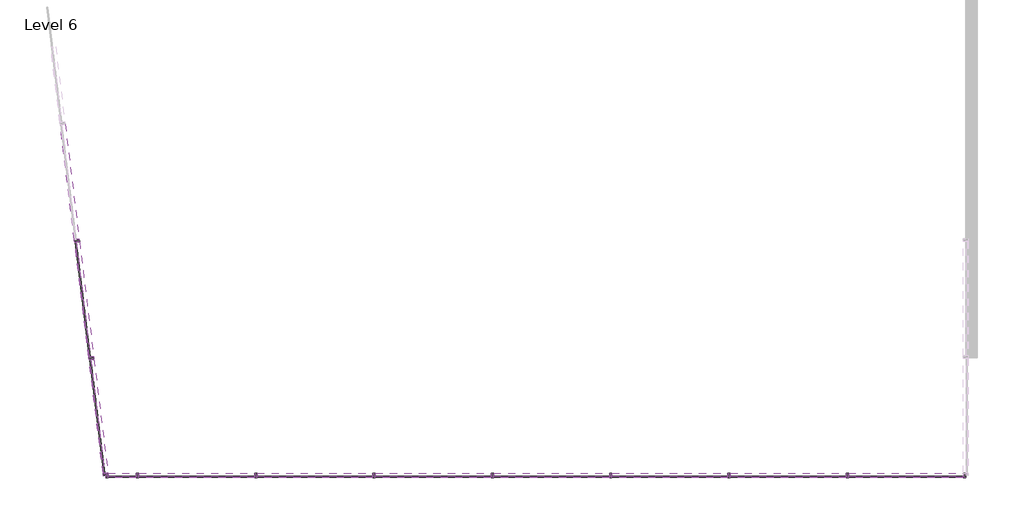
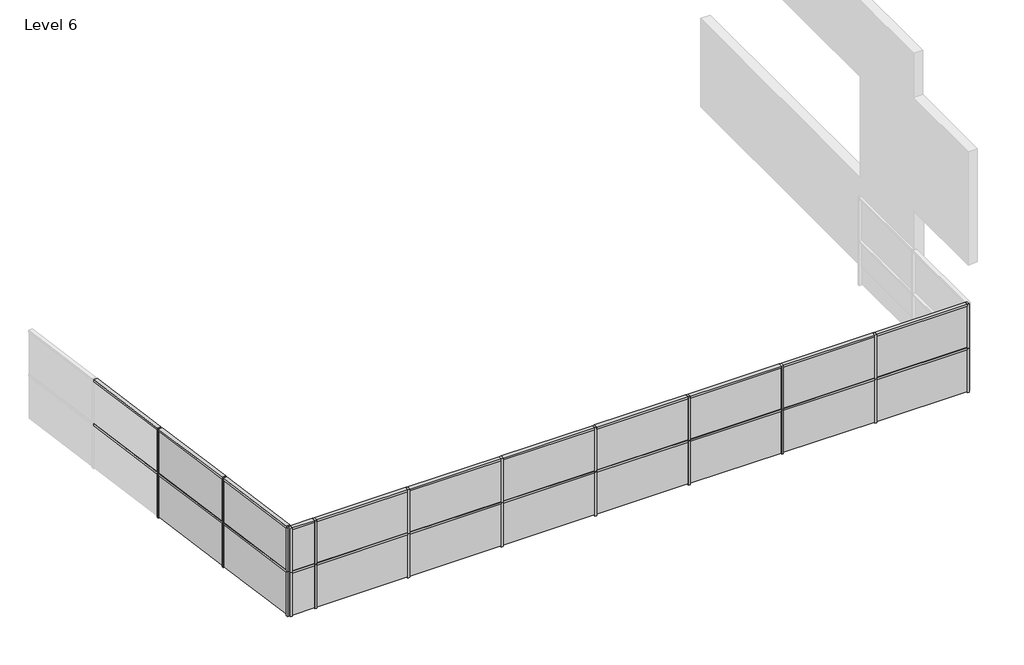
# One storey, part 1 of 2: 46 members, 20 plates.
"""IFC4 building model written with IfcOpenShell, lengths in millimetres."""

from ifc_helpers import new_model, si_unit, origin, place, context, project, spatial, transform, mapped, element, save
from components import member_daa7a266, member_82905deb, member_19d0a4ec, member_8cef0660, member_db480205, member_4491d118, member_0c11e56c, member_695b83e4, system_panel_glazed_37f15d2e, system_panel_glazed_3620f98e, system_panel_glazed_e46d4b42, system_panel_glazed_2a6c68b7, system_panel_glazed_07b088f8, system_panel_glazed_9d0e0944

model = new_model("IFC4")

# Units and contexts
model_context = context("Model", 3, world=origin())
ifc_project = project(units=[si_unit("LENGTHUNIT", "METRE", prefix="MILLI")], contexts=[model_context])

# Site, building, storey
site = spatial("IfcSite", under=ifc_project)
building = spatial("IfcBuilding", under=site)
storey = spatial("IfcBuildingStorey", under=building, Name="Level 6", Elevation=15240.0)

# Members
placement = place(None, origin())
member_shape = member_daa7a266(model_context)
element("IfcMember", 1, ObjectType="Rectangular Mullion : 2.5\" x 5\" rectangular", at=placement, inside=storey, context=model_context, shape_type="MappedRepresentation", body=[
    mapped(member_shape, transform((13839.0156363, -6979.1363705, 18288.0), x_axis=(0.0, 0.0, 1.0), y_axis=(0.0, -1.0, 0.0), z_axis=(1.0, 0.0, 0.0))),
])
member_2_shape = member_82905deb(model_context)
element("IfcMember", 2, ObjectType="Rectangular Mullion : 2.5\" x 5\" rectangular", at=placement, inside=storey, context=model_context, shape_type="MappedRepresentation", body=[
    mapped(member_2_shape, transform((10854.515636, -6979.1363705, 18288.0), x_axis=(-1.0, 0.0, 0.0), y_axis=(0.0, -1.0, 0.0), z_axis=(0.0, 0.0, 1.0))),
])
element("IfcMember", 3, ObjectType="Rectangular Mullion : 2.5\" x 5\" rectangular", at=placement, inside=storey, context=model_context, shape_type="MappedRepresentation", body=[
    mapped(member_2_shape, transform((7806.515636, -6979.1363705, 18288.0), x_axis=(-1.0, 0.0, 0.0), y_axis=(0.0, -1.0, 0.0), z_axis=(0.0, 0.0, 1.0))),
])
element("IfcMember", 4, ObjectType="Rectangular Mullion : 2.5\" x 5\" rectangular", at=placement, inside=storey, context=model_context, shape_type="MappedRepresentation", body=[
    mapped(member_2_shape, transform((4758.515636, -6979.1363705, 18288.0), x_axis=(-1.0, 0.0, 0.0), y_axis=(0.0, -1.0, 0.0), z_axis=(0.0, 0.0, 1.0))),
])
element("IfcMember", 5, ObjectType="Rectangular Mullion : 2.5\" x 5\" rectangular", at=placement, inside=storey, context=model_context, shape_type="MappedRepresentation", body=[
    mapped(member_2_shape, transform((1710.515636, -6979.1363705, 18288.0), x_axis=(-1.0, 0.0, 0.0), y_axis=(0.0, -1.0, 0.0), z_axis=(0.0, 0.0, 1.0))),
])
element("IfcMember", 6, ObjectType="Rectangular Mullion : 2.5\" x 5\" rectangular", at=placement, inside=storey, context=model_context, shape_type="MappedRepresentation", body=[
    mapped(member_2_shape, transform((-1337.484364, -6979.1363705, 18288.0), x_axis=(-1.0, 0.0, 0.0), y_axis=(0.0, -1.0, 0.0), z_axis=(0.0, 0.0, 1.0))),
])
element("IfcMember", 7, ObjectType="Rectangular Mullion : 2.5\" x 5\" rectangular", at=placement, inside=storey, context=model_context, shape_type="MappedRepresentation", body=[
    mapped(member_2_shape, transform((-4385.484364, -6979.1363705, 18288.0), x_axis=(-1.0, 0.0, 0.0), y_axis=(0.0, -1.0, 0.0), z_axis=(0.0, 0.0, 1.0))),
])
element("IfcMember", 8, ObjectType="Rectangular Mullion : 2.5\" x 5\" rectangular", at=placement, inside=storey, context=model_context, shape_type="MappedRepresentation", body=[
    mapped(member_2_shape, transform((-7433.484364, -6979.1363705, 18288.0), x_axis=(-1.0, 0.0, 0.0), y_axis=(0.0, -1.0, 0.0), z_axis=(0.0, 0.0, 1.0))),
])
member_3_shape = member_19d0a4ec(model_context)
element("IfcMember", 9, ObjectType="Rectangular Mullion : 2.5\" x 5\" rectangular", at=placement, inside=storey, context=model_context, shape_type="MappedRepresentation", body=[
    mapped(member_3_shape, transform((13839.0156363, -6979.1363705, 16764.0), x_axis=(0.0, 0.0, 1.0), y_axis=(0.0, -1.0, 0.0), z_axis=(1.0, 0.0, 0.0))),
])
element("IfcMember", 10, ObjectType="Rectangular Mullion : 2.5\" x 5\" rectangular", at=placement, inside=storey, context=model_context, shape_type="MappedRepresentation", body=[
    mapped(member_3_shape, transform((-8260.4765148, -6916.1096898, 16764.0), x_axis=(0.0, 0.0, 1.0), y_axis=(-0.9925461516413222, -0.12186934340514598, 0.0), z_axis=(0.12186934340514596, -0.9925461516413221, 0.0))),
])
element("IfcMember", 11, ObjectType="Rectangular Mullion : 2.5\" x 5\" rectangular", at=placement, inside=storey, context=model_context, shape_type="MappedRepresentation", body=[
    mapped(member_3_shape, transform((-8260.4765148, -6916.1096898, 18288.0), x_axis=(0.0, 0.0, 1.0), y_axis=(-0.9925461516413222, -0.12186934340514585, 0.0), z_axis=(0.12186934340514584, -0.9925461516413221, 0.0))),
])
member_4_shape = member_8cef0660(model_context)
element("IfcMember", 12, ObjectType="Rectangular Mullion : 2.5\" x 5\" rectangular", at=placement, inside=storey, context=model_context, shape_type="MappedRepresentation", body=[
    mapped(member_4_shape, transform((10822.765636, -6979.1363705, 16764.0), x_axis=(0.0, 0.0, 1.0), y_axis=(0.0, -1.0, 0.0), z_axis=(1.0, 0.0, 0.0))),
])
element("IfcMember", 13, ObjectType="Rectangular Mullion : 2.5\" x 5\" rectangular", at=placement, inside=storey, context=model_context, shape_type="MappedRepresentation", body=[
    mapped(member_4_shape, transform((7774.765636, -6979.1363705, 16764.0), x_axis=(0.0, 0.0, 1.0), y_axis=(0.0, -1.0, 0.0), z_axis=(1.0, 0.0, 0.0))),
])
element("IfcMember", 14, ObjectType="Rectangular Mullion : 2.5\" x 5\" rectangular", at=placement, inside=storey, context=model_context, shape_type="MappedRepresentation", body=[
    mapped(member_4_shape, transform((4726.765636, -6979.1363705, 16764.0), x_axis=(0.0, 0.0, 1.0), y_axis=(0.0, -1.0, 0.0), z_axis=(1.0, 0.0, 0.0))),
])
element("IfcMember", 15, ObjectType="Rectangular Mullion : 2.5\" x 5\" rectangular", at=placement, inside=storey, context=model_context, shape_type="MappedRepresentation", body=[
    mapped(member_4_shape, transform((1678.765636, -6979.1363705, 16764.0), x_axis=(0.0, 0.0, 1.0), y_axis=(0.0, -1.0, 0.0), z_axis=(1.0, 0.0, 0.0))),
])
element("IfcMember", 16, ObjectType="Rectangular Mullion : 2.5\" x 5\" rectangular", at=placement, inside=storey, context=model_context, shape_type="MappedRepresentation", body=[
    mapped(member_4_shape, transform((-1369.234364, -6979.1363705, 16764.0), x_axis=(0.0, 0.0, 1.0), y_axis=(0.0, -1.0, 0.0), z_axis=(1.0, 0.0, 0.0))),
])
element("IfcMember", 17, ObjectType="Rectangular Mullion : 2.5\" x 5\" rectangular", at=placement, inside=storey, context=model_context, shape_type="MappedRepresentation", body=[
    mapped(member_4_shape, transform((-4417.234364, -6979.1363705, 16764.0), x_axis=(0.0, 0.0, 1.0), y_axis=(0.0, -1.0, 0.0), z_axis=(1.0, 0.0, 0.0))),
])
element("IfcMember", 18, ObjectType="Rectangular Mullion : 2.5\" x 5\" rectangular", at=placement, inside=storey, context=model_context, shape_type="MappedRepresentation", body=[
    mapped(member_4_shape, transform((-8628.0649219, -3922.3423596, 16764.0), x_axis=(0.0, 0.0, 1.0), y_axis=(-0.9925461516413222, -0.12186934340514595, 0.0), z_axis=(0.12186934340514595, -0.9925461516413222, 0.0))),
])
element("IfcMember", 19, ObjectType="Rectangular Mullion : 2.5\" x 5\" rectangular", at=placement, inside=storey, context=model_context, shape_type="MappedRepresentation", body=[
    mapped(member_4_shape, transform((-8999.5226806, -897.0616894, 16764.0), x_axis=(0.0, 0.0, 1.0), y_axis=(-0.9925461516413222, -0.12186934340514602, 0.0), z_axis=(0.12186934340514602, -0.9925461516413222, 0.0))),
])
element("IfcMember", 20, ObjectType="Rectangular Mullion : 2.5\" x 5\" rectangular", at=placement, inside=storey, context=model_context, shape_type="MappedRepresentation", body=[
    mapped(member_4_shape, transform((-8628.0649219, -3922.3423596, 18288.0), x_axis=(0.0, 0.0, 1.0), y_axis=(-0.9925461516413222, -0.12186934340514595, 0.0), z_axis=(0.12186934340514595, -0.9925461516413222, 0.0))),
])
element("IfcMember", 21, ObjectType="Rectangular Mullion : 2.5\" x 5\" rectangular", at=placement, inside=storey, context=model_context, shape_type="MappedRepresentation", body=[
    mapped(member_4_shape, transform((-8999.5226806, -897.0616894, 18288.0), x_axis=(0.0, 0.0, 1.0), y_axis=(-0.9925461516413222, -0.12186934340514566, 0.0), z_axis=(0.12186934340514566, -0.9925461516413222, 0.0))),
])
member_5_shape = member_db480205(model_context)
element("IfcMember", 22, ObjectType="Rectangular Mullion : 2.5\" x 5\" rectangular", at=placement, inside=storey, context=model_context, shape_type="MappedRepresentation", body=[
    mapped(member_5_shape, transform((10822.765636, -6979.1363705, 18288.0), x_axis=(0.0, 0.0, 1.0), y_axis=(0.0, -1.0, 0.0), z_axis=(1.0, 0.0, 0.0))),
])
element("IfcMember", 23, ObjectType="Rectangular Mullion : 2.5\" x 5\" rectangular", at=placement, inside=storey, context=model_context, shape_type="MappedRepresentation", body=[
    mapped(member_5_shape, transform((7774.765636, -6979.1363705, 18288.0), x_axis=(0.0, 0.0, 1.0), y_axis=(0.0, -1.0, 0.0), z_axis=(1.0, 0.0, 0.0))),
])
element("IfcMember", 24, ObjectType="Rectangular Mullion : 2.5\" x 5\" rectangular", at=placement, inside=storey, context=model_context, shape_type="MappedRepresentation", body=[
    mapped(member_5_shape, transform((4726.765636, -6979.1363705, 18288.0), x_axis=(0.0, 0.0, 1.0), y_axis=(0.0, -1.0, 0.0), z_axis=(1.0, 0.0, 0.0))),
])
element("IfcMember", 25, ObjectType="Rectangular Mullion : 2.5\" x 5\" rectangular", at=placement, inside=storey, context=model_context, shape_type="MappedRepresentation", body=[
    mapped(member_5_shape, transform((1678.765636, -6979.1363705, 18288.0), x_axis=(0.0, 0.0, 1.0), y_axis=(0.0, -1.0, 0.0), z_axis=(1.0, 0.0, 0.0))),
])
element("IfcMember", 26, ObjectType="Rectangular Mullion : 2.5\" x 5\" rectangular", at=placement, inside=storey, context=model_context, shape_type="MappedRepresentation", body=[
    mapped(member_5_shape, transform((-1369.234364, -6979.1363705, 18288.0), x_axis=(0.0, 0.0, 1.0), y_axis=(0.0, -1.0, 0.0), z_axis=(1.0, 0.0, 0.0))),
])
element("IfcMember", 27, ObjectType="Rectangular Mullion : 2.5\" x 5\" rectangular", at=placement, inside=storey, context=model_context, shape_type="MappedRepresentation", body=[
    mapped(member_5_shape, transform((-4417.234364, -6979.1363705, 18288.0), x_axis=(0.0, 0.0, 1.0), y_axis=(0.0, -1.0, 0.0), z_axis=(1.0, 0.0, 0.0))),
])
element("IfcMember", 28, ObjectType="Rectangular Mullion : 2.5\" x 5\" rectangular", at=placement, inside=storey, context=model_context, shape_type="MappedRepresentation", body=[
    mapped(member_2_shape, transform((10854.515636, -6979.1363705, 16764.0), x_axis=(-1.0, 0.0, 0.0), y_axis=(0.0, -1.0, 0.0), z_axis=(0.0, 0.0, 1.0))),
])
element("IfcMember", 29, ObjectType="Rectangular Mullion : 2.5\" x 5\" rectangular", at=placement, inside=storey, context=model_context, shape_type="MappedRepresentation", body=[
    mapped(member_2_shape, transform((7806.515636, -6979.1363705, 16764.0), x_axis=(-1.0, 0.0, 0.0), y_axis=(0.0, -1.0, 0.0), z_axis=(0.0, 0.0, 1.0))),
])
element("IfcMember", 30, ObjectType="Rectangular Mullion : 2.5\" x 5\" rectangular", at=placement, inside=storey, context=model_context, shape_type="MappedRepresentation", body=[
    mapped(member_2_shape, transform((4758.515636, -6979.1363705, 16764.0), x_axis=(-1.0, 0.0, 0.0), y_axis=(0.0, -1.0, 0.0), z_axis=(0.0, 0.0, 1.0))),
])
element("IfcMember", 31, ObjectType="Rectangular Mullion : 2.5\" x 5\" rectangular", at=placement, inside=storey, context=model_context, shape_type="MappedRepresentation", body=[
    mapped(member_2_shape, transform((1710.515636, -6979.1363705, 16764.0), x_axis=(-1.0, 0.0, 0.0), y_axis=(0.0, -1.0, 0.0), z_axis=(0.0, 0.0, 1.0))),
])
element("IfcMember", 32, ObjectType="Rectangular Mullion : 2.5\" x 5\" rectangular", at=placement, inside=storey, context=model_context, shape_type="MappedRepresentation", body=[
    mapped(member_2_shape, transform((-1337.484364, -6979.1363705, 16764.0), x_axis=(-1.0, 0.0, 0.0), y_axis=(0.0, -1.0, 0.0), z_axis=(0.0, 0.0, 1.0))),
])
element("IfcMember", 33, ObjectType="Rectangular Mullion : 2.5\" x 5\" rectangular", at=placement, inside=storey, context=model_context, shape_type="MappedRepresentation", body=[
    mapped(member_2_shape, transform((-4385.484364, -6979.1363705, 16764.0), x_axis=(-1.0, 0.0, 0.0), y_axis=(0.0, -1.0, 0.0), z_axis=(0.0, 0.0, 1.0))),
])
element("IfcMember", 34, ObjectType="Rectangular Mullion : 2.5\" x 5\" rectangular", at=placement, inside=storey, context=model_context, shape_type="MappedRepresentation", body=[
    mapped(member_2_shape, transform((-7433.484364, -6979.1363705, 16764.0), x_axis=(-1.0, 0.0, 0.0), y_axis=(0.0, -1.0, 0.0), z_axis=(0.0, 0.0, 1.0))),
])
element("IfcMember", 35, ObjectType="Rectangular Mullion : 2.5\" x 5\" rectangular", at=placement, inside=storey, context=model_context, shape_type="MappedRepresentation", body=[
    mapped(member_2_shape, transform((-8624.1955702, -3953.8557, 16764.0), x_axis=(-0.1218693434051459, 0.9925461516413222, 0.0), y_axis=(-0.9925461516413222, -0.1218693434051459, 0.0), z_axis=(0.0, 0.0, 1.0))),
])
element("IfcMember", 36, ObjectType="Rectangular Mullion : 2.5\" x 5\" rectangular", at=placement, inside=storey, context=model_context, shape_type="MappedRepresentation", body=[
    mapped(member_2_shape, transform((-8624.1955702, -3953.8557, 18288.0), x_axis=(-0.1218693434051459, 0.9925461516413222, 0.0), y_axis=(-0.9925461516413222, -0.1218693434051459, 0.0), z_axis=(0.0, 0.0, 1.0))),
])
element("IfcMember", 37, ObjectType="Rectangular Mullion : 2.5\" x 5\" rectangular", at=placement, inside=storey, context=model_context, shape_type="MappedRepresentation", body=[
    mapped(member_2_shape, transform((-8995.6533289, -928.5750297, 16764.0), x_axis=(-0.1218693434051459, 0.9925461516413222, 0.0), y_axis=(-0.9925461516413222, -0.1218693434051459, 0.0), z_axis=(0.0, 0.0, 1.0))),
])
element("IfcMember", 38, ObjectType="Rectangular Mullion : 2.5\" x 5\" rectangular", at=placement, inside=storey, context=model_context, shape_type="MappedRepresentation", body=[
    mapped(member_2_shape, transform((-8995.6533289, -928.5750297, 18288.0), x_axis=(-0.1218693434051459, 0.9925461516413222, 0.0), y_axis=(-0.9925461516413222, -0.1218693434051459, 0.0), z_axis=(0.0, 0.0, 1.0))),
])
member_6_shape = member_4491d118(model_context)
element("IfcMember", 39, ObjectType="Rectangular Mullion : 2.5\" x 5\" rectangular", at=placement, inside=storey, context=model_context, shape_type="MappedRepresentation", body=[
    mapped(member_6_shape, transform((-8252.7378115, -6979.1363705, 18288.0), x_axis=(-1.0, 0.0, 0.0), y_axis=(0.0, -1.0, 0.0), z_axis=(0.0, 0.0, 1.0))),
])
element("IfcMember", 40, ObjectType="Rectangular Mullion : 2.5\" x 5\" rectangular", at=placement, inside=storey, context=model_context, shape_type="MappedRepresentation", body=[
    mapped(member_6_shape, transform((13902.5156363, -6979.1363705, 15240.0), x_axis=(1.0, 0.0, 0.0), y_axis=(0.0, -1.0, 0.0), z_axis=(0.0, 0.0, -1.0))),
])
element("IfcMember", 41, ObjectType="Rectangular Mullion : 2.5\" x 5\" rectangular", at=placement, inside=storey, context=model_context, shape_type="MappedRepresentation", body=[
    mapped(member_6_shape, transform((-8252.7378115, -6979.1363705, 15240.0), x_axis=(0.1218693434051459, -0.9925461516413222, 0.0), y_axis=(-0.9925461516413222, -0.1218693434051459, 0.0), z_axis=(0.0, 0.0, -1.0))),
])
element("IfcMember", 42, ObjectType="Rectangular Mullion : 2.5\" x 5\" rectangular", at=placement, inside=storey, context=model_context, shape_type="MappedRepresentation", body=[
    mapped(member_6_shape, transform((-8252.7378115, -6979.1363705, 16764.0), x_axis=(0.1218693434051459, -0.9925461516413222, 0.0), y_axis=(-0.9925461516413222, -0.1218693434051459, 0.0), z_axis=(0.0, 0.0, -1.0))),
])
element("IfcMember", 43, ObjectType="Rectangular Mullion : 2.5\" x 5\" rectangular", at=placement, inside=storey, context=model_context, shape_type="MappedRepresentation", body=[
    mapped(member_6_shape, transform((13902.5156363, -6979.1363705, 16764.0), x_axis=(1.0, 0.0, 0.0), y_axis=(0.0, -1.0, 0.0), z_axis=(0.0, 0.0, -1.0))),
])
element("IfcMember", 44, ObjectType="Rectangular Mullion : 2.5\" x 5\" rectangular", at=placement, inside=storey, context=model_context, shape_type="MappedRepresentation", body=[
    mapped(member_6_shape, transform((-8252.7378115, -6979.1363705, 16764.0), x_axis=(-1.0, 0.0, 0.0), y_axis=(0.0, -1.0, 0.0), z_axis=(0.0, 0.0, 1.0))),
])
member_7_shape = member_0c11e56c(model_context)
element("IfcMember", 45, ObjectType="Rectangular Mullion : 2.5\" x 5\" rectangular", at=placement, inside=storey, context=model_context, shape_type="MappedRepresentation", body=[
    mapped(member_7_shape, transform((-7465.234364, -6979.1363705, 16764.0), x_axis=(0.0, 0.0, 1.0), y_axis=(0.0, -1.0, 0.0), z_axis=(1.0, 0.0, 0.0))),
])
member_8_shape = member_695b83e4(model_context)
element("IfcMember", 46, ObjectType="Rectangular Mullion : 2.5\" x 5\" rectangular", at=placement, inside=storey, context=model_context, shape_type="MappedRepresentation", body=[
    mapped(member_8_shape, transform((-7465.234364, -6979.1363705, 18288.0), x_axis=(0.0, 0.0, 1.0), y_axis=(0.0, -1.0, 0.0), z_axis=(1.0, 0.0, 0.0))),
])

# Plates
system_panel_glazed_shape = system_panel_glazed_37f15d2e(model_context)
element("IfcPlate", 47, ObjectType="System Panel : Glazed", at=placement, inside=storey, context=model_context, shape_type="MappedRepresentation", body=[
    mapped(system_panel_glazed_shape, transform((12362.6406361, -6979.1363705, 16795.75), x_axis=(-1.0, 0.0, 0.0), y_axis=(0.0, -1.0, 0.0), z_axis=(0.0, 0.0, 1.0))),
])
system_panel_glazed_2_shape = system_panel_glazed_3620f98e(model_context)
element("IfcPlate", 48, ObjectType="System Panel : Glazed", at=placement, inside=storey, context=model_context, shape_type="MappedRepresentation", body=[
    mapped(system_panel_glazed_2_shape, transform((9330.515636, -6979.1363705, 16795.75), x_axis=(-1.0, 0.0, 0.0), y_axis=(0.0, -1.0, 0.0), z_axis=(0.0, 0.0, 1.0))),
])
element("IfcPlate", 49, ObjectType="System Panel : Glazed", at=placement, inside=storey, context=model_context, shape_type="MappedRepresentation", body=[
    mapped(system_panel_glazed_2_shape, transform((6282.515636, -6979.1363705, 16795.75), x_axis=(-1.0, 0.0, 0.0), y_axis=(0.0, -1.0, 0.0), z_axis=(0.0, 0.0, 1.0))),
])
element("IfcPlate", 50, ObjectType="System Panel : Glazed", at=placement, inside=storey, context=model_context, shape_type="MappedRepresentation", body=[
    mapped(system_panel_glazed_2_shape, transform((3234.515636, -6979.1363705, 16795.75), x_axis=(-1.0, 0.0, 0.0), y_axis=(0.0, -1.0, 0.0), z_axis=(0.0, 0.0, 1.0))),
])
element("IfcPlate", 51, ObjectType="System Panel : Glazed", at=placement, inside=storey, context=model_context, shape_type="MappedRepresentation", body=[
    mapped(system_panel_glazed_2_shape, transform((186.515636, -6979.1363705, 16795.75), x_axis=(-1.0, 0.0, 0.0), y_axis=(0.0, -1.0, 0.0), z_axis=(0.0, 0.0, 1.0))),
])
element("IfcPlate", 52, ObjectType="System Panel : Glazed", at=placement, inside=storey, context=model_context, shape_type="MappedRepresentation", body=[
    mapped(system_panel_glazed_2_shape, transform((-2861.484364, -6979.1363705, 16795.75), x_axis=(-1.0, 0.0, 0.0), y_axis=(0.0, -1.0, 0.0), z_axis=(0.0, 0.0, 1.0))),
])
element("IfcPlate", 53, ObjectType="System Panel : Glazed", at=placement, inside=storey, context=model_context, shape_type="MappedRepresentation", body=[
    mapped(system_panel_glazed_2_shape, transform((-5909.484364, -6979.1363705, 16795.75), x_axis=(-1.0, 0.0, 0.0), y_axis=(0.0, -1.0, 0.0), z_axis=(0.0, 0.0, 1.0))),
])
system_panel_glazed_3_shape = system_panel_glazed_e46d4b42(model_context)
element("IfcPlate", 54, ObjectType="System Panel : Glazed", at=placement, inside=storey, context=model_context, shape_type="MappedRepresentation", body=[
    mapped(system_panel_glazed_3_shape, transform((12362.6406361, -6979.1363705, 15271.75), x_axis=(-1.0, 0.0, 0.0), y_axis=(0.0, -1.0, 0.0), z_axis=(0.0, 0.0, 1.0))),
])
element("IfcPlate", 55, ObjectType="System Panel : Glazed", at=placement, inside=storey, context=model_context, shape_type="MappedRepresentation", body=[
    mapped(system_panel_glazed_3_shape, transform((-8440.4013667, -5450.739365, 15271.75), x_axis=(-0.1218693434051459, 0.9925461516413222, 0.0), y_axis=(-0.9925461516413222, -0.1218693434051459, 0.0), z_axis=(0.0, 0.0, 1.0))),
])
element("IfcPlate", 56, ObjectType="System Panel : Glazed", at=placement, inside=storey, context=model_context, shape_type="MappedRepresentation", body=[
    mapped(system_panel_glazed_3_shape, transform((-8440.4013667, -5450.739365, 16795.75), x_axis=(-0.1218693434051459, 0.9925461516413222, 0.0), y_axis=(-0.9925461516413222, -0.1218693434051459, 0.0), z_axis=(0.0, 0.0, 1.0))),
])
system_panel_glazed_4_shape = system_panel_glazed_2a6c68b7(model_context)
element("IfcPlate", 57, ObjectType="System Panel : Glazed", at=placement, inside=storey, context=model_context, shape_type="MappedRepresentation", body=[
    mapped(system_panel_glazed_4_shape, transform((9330.515636, -6979.1363705, 15271.75), x_axis=(-1.0, 0.0, 0.0), y_axis=(0.0, -1.0, 0.0), z_axis=(0.0, 0.0, 1.0))),
])
element("IfcPlate", 58, ObjectType="System Panel : Glazed", at=placement, inside=storey, context=model_context, shape_type="MappedRepresentation", body=[
    mapped(system_panel_glazed_4_shape, transform((6282.515636, -6979.1363705, 15271.75), x_axis=(-1.0, 0.0, 0.0), y_axis=(0.0, -1.0, 0.0), z_axis=(0.0, 0.0, 1.0))),
])
element("IfcPlate", 59, ObjectType="System Panel : Glazed", at=placement, inside=storey, context=model_context, shape_type="MappedRepresentation", body=[
    mapped(system_panel_glazed_4_shape, transform((3234.515636, -6979.1363705, 15271.75), x_axis=(-1.0, 0.0, 0.0), y_axis=(0.0, -1.0, 0.0), z_axis=(0.0, 0.0, 1.0))),
])
element("IfcPlate", 60, ObjectType="System Panel : Glazed", at=placement, inside=storey, context=model_context, shape_type="MappedRepresentation", body=[
    mapped(system_panel_glazed_4_shape, transform((186.515636, -6979.1363705, 15271.75), x_axis=(-1.0, 0.0, 0.0), y_axis=(0.0, -1.0, 0.0), z_axis=(0.0, 0.0, 1.0))),
])
element("IfcPlate", 61, ObjectType="System Panel : Glazed", at=placement, inside=storey, context=model_context, shape_type="MappedRepresentation", body=[
    mapped(system_panel_glazed_4_shape, transform((-2861.484364, -6979.1363705, 15271.75), x_axis=(-1.0, 0.0, 0.0), y_axis=(0.0, -1.0, 0.0), z_axis=(0.0, 0.0, 1.0))),
])
element("IfcPlate", 62, ObjectType="System Panel : Glazed", at=placement, inside=storey, context=model_context, shape_type="MappedRepresentation", body=[
    mapped(system_panel_glazed_4_shape, transform((-5909.484364, -6979.1363705, 15271.75), x_axis=(-1.0, 0.0, 0.0), y_axis=(0.0, -1.0, 0.0), z_axis=(0.0, 0.0, 1.0))),
])
element("IfcPlate", 63, ObjectType="System Panel : Glazed", at=placement, inside=storey, context=model_context, shape_type="MappedRepresentation", body=[
    mapped(system_panel_glazed_4_shape, transform((-8809.9244496, -2441.2153649, 15271.75), x_axis=(-0.1218693434051459, 0.9925461516413222, 0.0), y_axis=(-0.9925461516413222, -0.1218693434051459, 0.0), z_axis=(0.0, 0.0, 1.0))),
])
element("IfcPlate", 64, ObjectType="System Panel : Glazed", at=placement, inside=storey, context=model_context, shape_type="MappedRepresentation", body=[
    mapped(system_panel_glazed_4_shape, transform((-8809.9244496, -2441.2153649, 16795.75), x_axis=(-0.1218693434051459, 0.9925461516413222, 0.0), y_axis=(-0.9925461516413222, -0.1218693434051459, 0.0), z_axis=(0.0, 0.0, 1.0))),
])
system_panel_glazed_5_shape = system_panel_glazed_07b088f8(model_context)
element("IfcPlate", 65, ObjectType="System Panel : Glazed", at=placement, inside=storey, context=model_context, shape_type="MappedRepresentation", body=[
    mapped(system_panel_glazed_5_shape, transform((-7827.2360878, -6979.1363705, 16795.75), x_axis=(-1.0, 0.0, 0.0), y_axis=(0.0, -1.0, 0.0), z_axis=(0.0, 0.0, 1.0))),
])
system_panel_glazed_6_shape = system_panel_glazed_9d0e0944(model_context)
element("IfcPlate", 66, ObjectType="System Panel : Glazed", at=placement, inside=storey, context=model_context, shape_type="MappedRepresentation", body=[
    mapped(system_panel_glazed_6_shape, transform((-7827.2360878, -6979.1363705, 15271.75), x_axis=(-1.0, 0.0, 0.0), y_axis=(0.0, -1.0, 0.0), z_axis=(0.0, 0.0, 1.0))),
])

save(model, "model.ifc")

# Revit data of these elements
# Type "Rectangular Mullion : 2.5\" x 5\" rectangular"
#   built-in parameter 1007304 = 0.416667 (stored number, unit not read)
#   built-in parameter 1007301 = 0.104167 (stored number, unit not read)
#   built-in parameter 1007300 = 0.104167 (stored number, unit not read)
# Type "System Panel : Glazed"
#   Construction Type Id = "GSP4R"
#   Analytic Construction = "1/8 in Pilkington single glazing"
#   Visual Light Transmittance = 0.9
#   Solar Heat Gain Coefficient = 0.86
#   Heat Transfer Coefficient (U) = 1.18115 BTU/(h·ft²·°F)
#   Define Thermal Properties by = 1
# Elements 1, 2, 3, 4, 5, 6, 7, 8, 9, 10, 11, 12, 13, 14, 15, 16, 17, 18, 19, 20, 21, 22, 23, 24, 25, 26, 27, 28, 29, 30, 31, 32, 33, 34, 35, 36, 37, 38, 39, 40, 41, 42, 43, 44, 45, 46 (IfcMember, "Rectangular Mullion : 2.5\" x 5\" rectangular")
#   Phase Created = New Construction
#   Materials on its faces: "Aluminum"
# Elements 47, 48, 49, 50, 51, 52, 53, 54, 55, 56, 57, 58, 59, 60, 61, 62, 63, 64, 65, 66 (IfcPlate, "System Panel : Glazed")
#   Phase Created = New Construction
#   Materials on its faces: "Glass"
# Materials
#   "Aluminum": class "Metal", colour RGB 247 247 247, transparency 0, Description = "Aluminum 6061", Cost = 0
#   "Glass": class "Glass", colour RGB 0 128 192, transparency 0.75, Description = "Soda Lime Glass", Cost = 0
